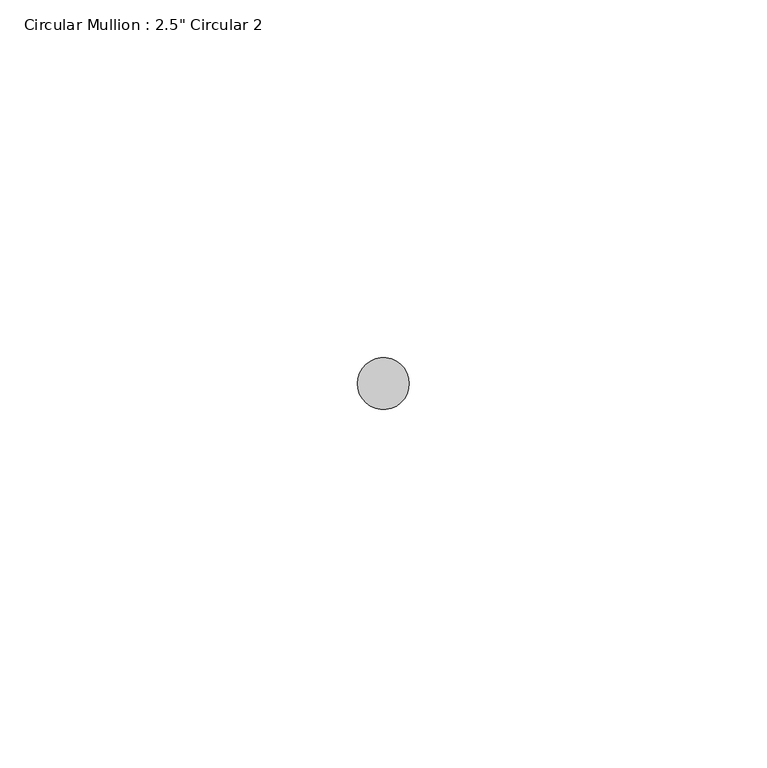
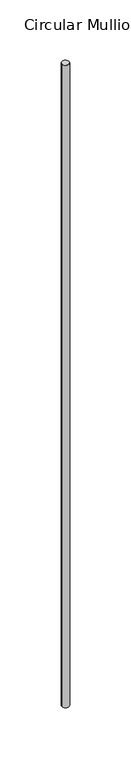
"""IFC4 building model written with IfcOpenShell, lengths in millimetres: member geometry."""

from ifc_helpers import new_model, si_unit, point, frame, origin, origin_2d, place, context, project, spatial, circle_curve, trimmed, segment, composite_curve, outline, extrude, source, transform, mapped, element, save


def member_4e015be9(model_context):
    return source(origin(), model_context, "Body", "SweptSolid", [
        extrude(outline(composite_curve([segment(trimmed(circle_curve(origin_2d(), 3.6195), [point((3.6195, 0.0))], [point((-3.6195, 0.0))], False, "CARTESIAN"), True, "CONTINUOUS"), segment(trimmed(circle_curve(origin_2d(), 3.6195), [point((-3.6195, 0.0))], [point((3.6195, 0.0))], False, "CARTESIAN"), True, "CONTINUOUS")], self_intersect=False)), frame((0.0, 0.0, -659.511), z_axis=(0.0, 0.0, 1.0), x_axis=(1.0, 0.0, 0.0)), (0.0, 0.0, 1.0), 659.511),
    ])


if __name__ == "__main__":
    model = new_model("IFC4")
    model_context = context("Model", 3, world=origin())
    ifc_project = project(units=[si_unit("LENGTHUNIT", "METRE", prefix="MILLI")], contexts=[model_context])
    site = spatial("IfcSite", under=ifc_project)
    building = spatial("IfcBuilding", under=site)
    placement = place(None, origin())
    member_shape = member_4e015be9(model_context)
    element("IfcMember", 1, ObjectType="Circular Mullion : 2.5\" Circular 2", at=placement, inside=building, context=model_context, shape_type="MappedRepresentation", body=[
        mapped(member_shape, transform((0.0, 0.0, 0.0), x_axis=(1.0, 0.0, 0.0), y_axis=(0.0, 1.0, 0.0), z_axis=(0.0, 0.0, 1.0))),
    ])
    save(model, "model.ifc")

# Revit data of these elements
# Type "Circular Mullion : 2.5\" Circular 2"
#   built-in parameter 1007350 = 0.011875 (stored number, unit not read)
# Element 1 (IfcMember, "Circular Mullion : 2.5\" Circular 2")
#   Materials on its faces: "Aluminum"
# Materials
#   "Aluminum": class "Metal", colour RGB 247 247 247, transparency 0, Description = "Aluminum 6061", Cost = 0
